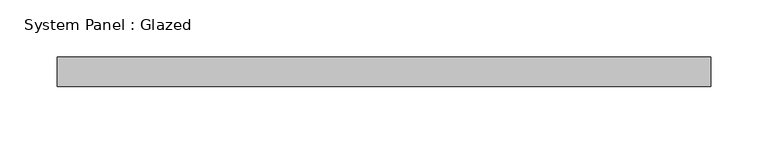
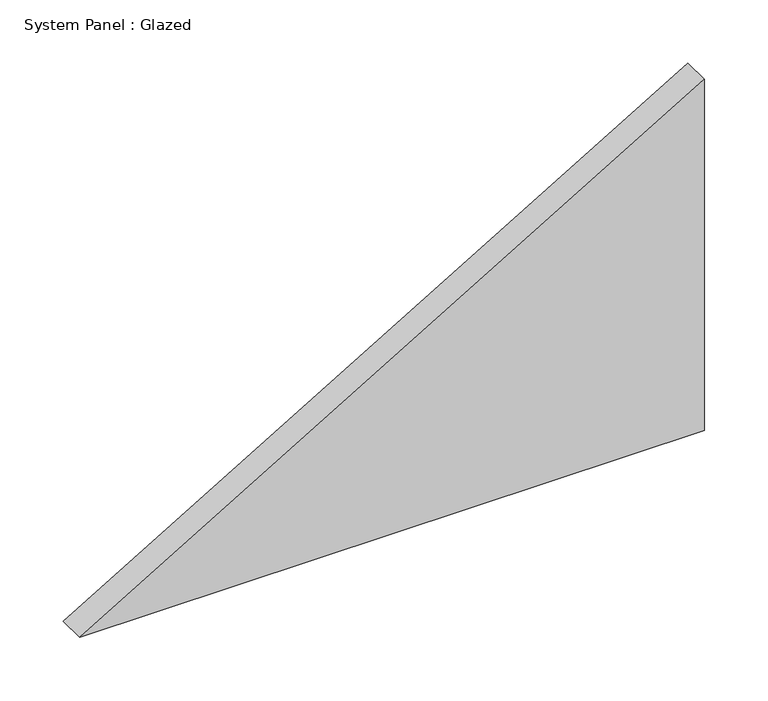
"""IFC4 building model written with IfcOpenShell, lengths in millimetres: plate geometry, System Panel : Glazed."""

from ifc_helpers import new_model, si_unit, frame, origin, place, context, project, spatial, polyline, outline, extrude, source, transform, mapped, element, save


def system_panel_glazed_28184e5f(model_context):
    return source(origin(), model_context, "Body", "SweptSolid", [
        extrude(outline(polyline([(0.0, -284.3459491), (0.0, 284.3459491), (337.9987292, 284.3459491), (0.0, -284.3459491)])), frame((0.0, 19.05, 0.0), z_axis=(0.0, 1.0, 0.0), x_axis=(0.0, 0.0, 1.0)), (0.0, 0.0, 1.0), 25.4),
    ])


if __name__ == "__main__":
    model = new_model("IFC4")
    model_context = context("Model", 3, world=origin())
    ifc_project = project(units=[si_unit("LENGTHUNIT", "METRE", prefix="MILLI")], contexts=[model_context])
    site = spatial("IfcSite", under=ifc_project)
    building = spatial("IfcBuilding", under=site)
    placement = place(None, origin())
    system_panel_glazed_shape = system_panel_glazed_28184e5f(model_context)
    element("IfcPlate", 1, ObjectType="System Panel : Glazed", at=placement, inside=building, context=model_context, shape_type="MappedRepresentation", body=[
        mapped(system_panel_glazed_shape, transform((0.0, 0.0, 0.0), x_axis=(1.0, 0.0, 0.0), y_axis=(0.0, 1.0, 0.0), z_axis=(0.0, 0.0, 1.0))),
    ])
    save(model, "model.ifc")

# Revit data of these elements
# Type "System Panel : Glazed"
#   Construction Type Id = "GSP4R"
#   Analytic Construction = "1/8 in Pilkington single glazing"
#   Visual Light Transmittance = 0.9
#   Solar Heat Gain Coefficient = 0.86
#   Heat Transfer Coefficient (U) = 1.18115 BTU/(h·ft²·°F)
#   Define Thermal Properties by = 1
# Element 1 (IfcPlate, "System Panel : Glazed")
#   Materials on its faces: "Glass"
# Materials
#   "Glass": class "Glass", colour RGB 0 128 192, transparency 0.75, Description = "Soda Lime Glass", Cost = 0
